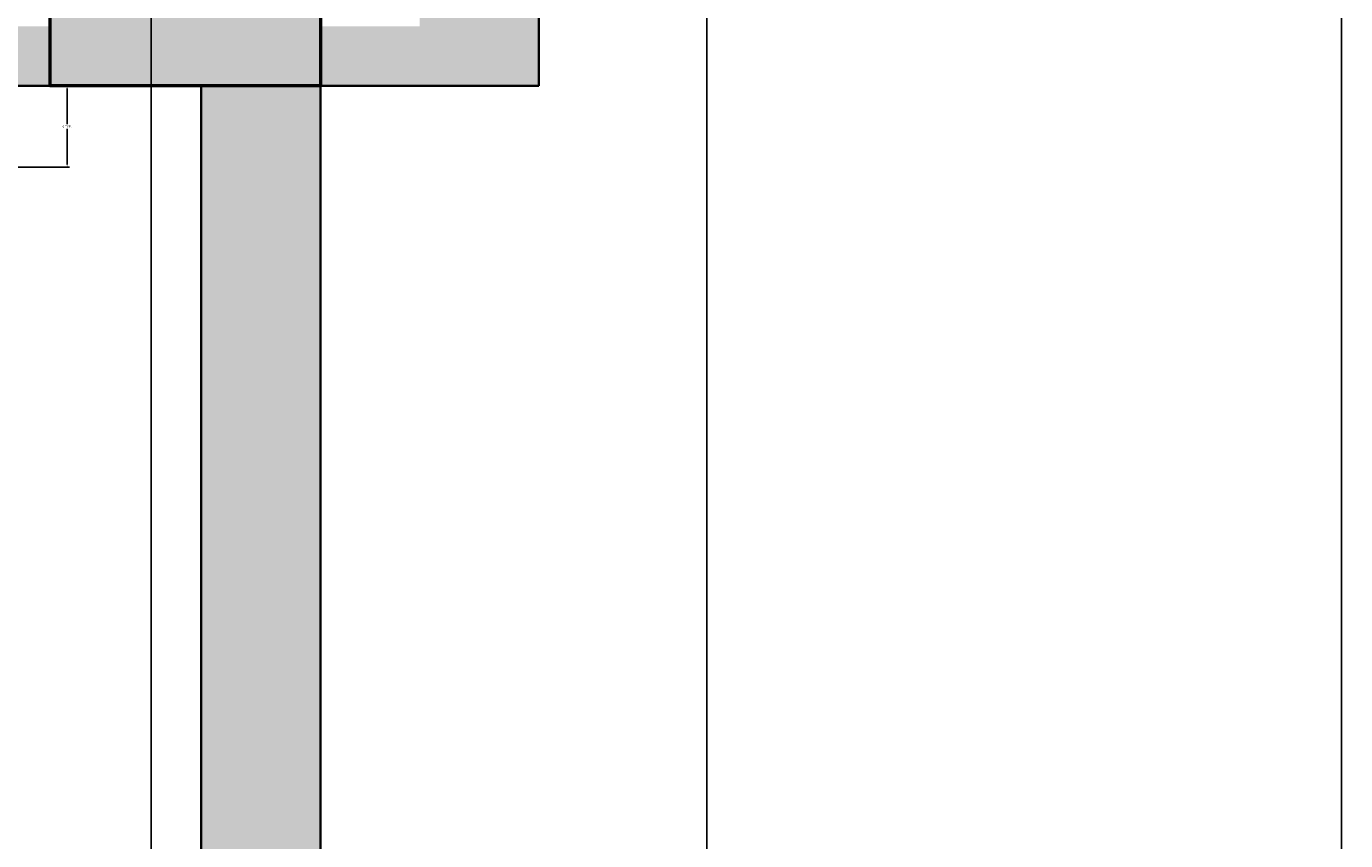
# Model space of a CAD drawing. Units: inches. Extents: x 1998 to 2588, y 1139 to 1977.
# Tile 133 of 134: x 2489 to 2588, y 1698 to 1760. Entities that reach past the tile are written whole.
import ezdxf

# ---------------------------------------------------------------- set-up
doc = ezdxf.new("R2010")
doc.units = ezdxf.units.IN
for name, color, linetype, lineweight in [('A-ANNO-DIMS', 2, 'Continuous', 18), ('A-COLS-PATT', 250, 'Continuous', 13), ('A-WALL-PATT', 252, 'Continuous', 13), ('COLUMN', 10, 'Continuous', 50), ('WALL', 200, 'Continuous', 35)]:
    doc.layers.add(name, color=color, linetype=linetype, lineweight=lineweight)
doc.styles.get("Standard").update_dxf_attribs({"font": 'arial.ttf'})
doc.dimstyles.get("Standard").update_dxf_attribs({"dimtxt": 0.18, "dimasz": 0.18, "dimexe": 0.18, "dimexo": 0.0625, "dimgap": 0.09, "dimtad": 0, "dimtih": 1, "dimtoh": 1, "dimdec": 4, "dimzin": 0, "dimdsep": 46, "dimtxsty": 'Standard', "dimcen": 0.09, "dimadec": 0, "dimazin": 0, "dimtfac": 1, "dimtdec": 4, "dimtofl": 0, "dimtmove": 0, "dimatfit": 3, "dimfxl": 1, "dimtolj": 1, "dimtzin": 0, "dimarcsym": 0})

# ---------------------------------------------------------------- blocks, each defined once
blk = doc.blocks.new('*D18')
at = {"layer": 'A-ANNO-DIMS', "color": 0, "lineweight": -2, "transparency": 16777216}
for p, q in [((2481.104, 1755.232), (2492.018, 1755.232)), ((2491.838, 1755.052), (2491.838, 1752.353)), ((2491.838, 1749.289), (2491.838, 1751.989)), ((2481.104, 1749.109), (2492.018, 1749.109))]:
    blk.add_line(p, q, dxfattribs=at)
at = {"layer": 'A-ANNO-DIMS', "color": 0, "transparency": 16777216}
for points in [[(2491.808, 1755.052), (2491.868, 1755.052), (2491.838, 1755.232)], [(2491.808, 1749.289), (2491.868, 1749.289), (2491.838, 1749.109)]]:
    blk.add_solid(points, dxfattribs=at)
at = {"layer": 'Defpoints', "color": 0, "transparency": 16777216}
for p in [(2481.042, 1755.232), (2491.838, 1755.232), (2481.042, 1749.109)]:
    blk.add_point(p, dxfattribs=at)
at = {"layer": 'A-ANNO-DIMS', "color": 0, "transparency": 16777216, "insert": (2491.838, 1752.171), "char_height": 0.18, "attachment_point": 5}
blk.add_mtext('\\A1;6 TYP.', dxfattribs=at)
blk = doc.blocks.new('*D24')
at = {"layer": 'A-ANNO-DIMS', "color": 0, "lineweight": -2, "transparency": 16777216}
for p, q in [((2398.535, 1911.232), (2588.309, 1911.232)), ((2588.129, 1911.052), (2588.129, 1570.164)), ((2588.129, 1228.912), (2588.129, 1569.8)), ((2527.535, 1228.732), (2588.309, 1228.732))]:
    blk.add_line(p, q, dxfattribs=at)
at = {"layer": 'A-ANNO-DIMS', "color": 0, "transparency": 16777216}
for points in [[(2588.099, 1911.052), (2588.159, 1911.052), (2588.129, 1911.232)], [(2588.099, 1228.912), (2588.159, 1228.912), (2588.129, 1228.732)]]:
    blk.add_solid(points, dxfattribs=at)
at = {"layer": 'Defpoints', "color": 0, "transparency": 16777216}
for p in [(2398.473, 1911.232), (2588.129, 1911.232), (2527.473, 1228.732)]:
    blk.add_point(p, dxfattribs=at)
at = {"layer": 'A-ANNO-DIMS', "color": 0, "transparency": 16777216, "insert": (2588.129, 1569.982), "char_height": 0.18, "attachment_point": 5}
blk.add_mtext('\\A1;682.5', dxfattribs=at)
blk = doc.blocks.new('*D31')
at = {"layer": 'A-ANNO-DIMS', "color": 0, "lineweight": -2, "transparency": 16777216}
for p, q in [((2498.179, 1636.795), (2498.179, 1977.362)), ((2498.359, 1977.182), (2518.957, 1977.182)), ((2539.999, 1977.182), (2519.4, 1977.182)), ((2540.179, 1636.795), (2540.179, 1977.362))]:
    blk.add_line(p, q, dxfattribs=at)
at = {"layer": 'A-ANNO-DIMS', "color": 0, "transparency": 16777216}
for points in [[(2498.359, 1977.212), (2498.359, 1977.152), (2498.179, 1977.182)], [(2539.999, 1977.212), (2539.999, 1977.152), (2540.179, 1977.182)]]:
    blk.add_solid(points, dxfattribs=at)
at = {"layer": 'Defpoints', "color": 0, "transparency": 16777216}
for p in [(2540.179, 1977.182), (2498.179, 1636.732), (2540.179, 1636.732)]:
    blk.add_point(p, dxfattribs=at)
at = {"layer": 'A-ANNO-DIMS', "color": 0, "transparency": 16777216, "insert": (2519.179, 1977.182), "char_height": 0.18, "attachment_point": 5}
blk.add_mtext('\\A1;42', dxfattribs=at)

msp = doc.modelspace()

# ---------------------------------------------------------------- hatches: boundary and pattern name
at = {"layer": 'A-COLS-PATT'}
h = msp.add_hatch(color=256, dxfattribs=at)
h.dxf.hatch_style = 1
h.paths.add_polyline_path([(2099.4125, 1888.7324), (2087.9729, 1888.7324), (2087.9729, 1868.3278), (2099.4125, 1868.3278)])
h.paths.add_polyline_path([(2234.4125, 1888.7324), (2222.9729, 1888.7324), (2222.9729, 1868.3278), (2234.4125, 1868.3278)])
h.paths.add_polyline_path([(2341.4729, 1886.637), (2330.0332, 1886.637), (2330.0332, 1866.2324), (2341.4729, 1866.2324)])
h.paths.add_polyline_path([(2507.8006, 1882.7324), (2487.396, 1882.7324), (2487.396, 1871.2927), (2507.8006, 1871.2927)])
h.paths.add_polyline_path([(2510.9729, 1766.672), (2490.5682, 1766.672), (2490.5682, 1755.2324), (2510.9729, 1755.2324)])
h.paths.add_polyline_path([(2345.9729, 1759.7324), (2334.5332, 1759.7324), (2334.5332, 1739.3278), (2345.9729, 1739.3278)])
h.paths.add_polyline_path([(2234.4125, 1774.3318), (2222.9729, 1774.3318), (2222.9729, 1753.9272), (2234.4125, 1753.9272)])
h.paths.add_polyline_path([(2099.4125, 1775.637), (2087.9729, 1775.637), (2087.9729, 1755.2324), (2099.4125, 1755.2324)])
h.paths.add_polyline_path([(2098.0956, 1593.7241), (2077.691, 1593.7241), (2077.691, 1582.2845), (2098.0956, 1582.2845)])
h.paths.add_polyline_path([(2227.4729, 1604.637), (2216.0332, 1604.637), (2216.0332, 1584.2324), (2227.4729, 1584.2324)])
h.paths.add_polyline_path([(2345.9729, 1647.5211), (2334.5332, 1647.5211), (2334.5332, 1627.1165), (2345.9729, 1627.1165)])
h.paths.add_polyline_path([(2522.3775, 1641.2324), (2501.9729, 1641.2324), (2501.9729, 1629.7927), (2522.3775, 1629.7927)])
h.paths.add_polyline_path([(2522.3775, 1480.7324), (2501.9729, 1480.7324), (2501.9729, 1469.2927), (2522.3775, 1469.2927)])
h.paths.add_polyline_path([(2345.9729, 1488.5616), (2334.5332, 1488.5616), (2334.5332, 1468.1569), (2345.9729, 1468.1569)])
h.paths.add_polyline_path([(2234.4125, 1486.137), (2227.4729, 1486.137), (2227.4729, 1465.7324), (2234.4125, 1465.7324)])
h.paths.add_polyline_path([(2227.4729, 1486.137), (2222.9729, 1486.137), (2222.9729, 1465.7324), (2227.4729, 1465.7324)])
h.paths.add_polyline_path([(2108.3775, 1470.2324), (2087.9729, 1470.2324), (2087.9729, 1458.7927), (2108.3775, 1458.7927)])
h.paths.add_polyline_path([(2096.9729, 1365.5012), (2087.9729, 1365.5012), (2087.9729, 1345.0966), (2096.9729, 1345.0966)])
h.paths.add_polyline_path([(2087.9729, 1365.5012), (2085.5332, 1365.5012), (2085.5332, 1345.0966), (2087.9729, 1345.0966)])
h.paths.add_polyline_path([(2234.4125, 1285.137), (2222.9729, 1285.137), (2222.9729, 1264.7324), (2234.4125, 1264.7324)])
h.paths.add_polyline_path([(2345.9729, 1285.137), (2334.5332, 1285.137), (2334.5332, 1264.7324), (2345.9729, 1264.7324)])
h.paths.add_polyline_path([(2503.1458, 1240.172), (2482.7412, 1240.172), (2482.7412, 1228.7324), (2503.1458, 1228.7324)])
h.paths.add_polyline_path([(2510.9729, 1369.172), (2490.5682, 1369.172), (2490.5682, 1357.7324), (2510.9729, 1357.7324)])
at = {"layer": 'A-WALL-PATT'}
h = msp.add_hatch(color=256, dxfattribs=at)
h.dxf.hatch_style = 1
h.paths.add_polyline_path([(2227.4729, 1911.2324), (2222.9729, 1911.2324), (2222.9729, 1888.7324), (2227.4729, 1888.7324)])
h.paths.add_polyline_path([(2236.4493, 1870.3636), (2236.4493, 1875.2324), (2234.4125, 1875.2324), (2234.4125, 1868.3278), (2227.4729, 1868.3278), (2227.4729, 1866.2324), (2236.4493, 1866.2324)])
h.paths.add_polyline_path([(2330.0332, 1875.2324), (2263.9907, 1875.2324), (2263.9907, 1866.2324), (2330.0332, 1866.2324)])
h.paths.add_polyline_path([(2345.9729, 1906.7324), (2393.9729, 1906.7324), (2393.9729, 1882.7324), (2345.9729, 1882.7324), (2345.9729, 1878.2324), (2393.9729, 1878.2324), (2398.4729, 1878.2324), (2398.4729, 1882.7324), (2398.4729, 1911.2324), (2345.9729, 1911.2324), (2341.4729, 1911.2324), (2341.4729, 1866.2324), (2341.4729, 1790.0412), (2345.9729, 1790.0412), (2345.9729, 1875.2324)])
h.paths.add_polyline_path([(2398.4729, 1878.2324), (2393.9729, 1878.2324), (2393.9729, 1798.2324), (2393.9729, 1793.7324), (2398.4729, 1793.7324)], flags=17)
h.paths.add_polyline_path([(2393.9729, 1798.2324), (2375.7311, 1798.2324, -0.005968), (2375.7384, 1797.6146), (2375.7384, 1793.7324), (2393.9729, 1793.7324)], flags=17)
h.paths.add_polyline_path([(2349.8569, 1797.6146), (2349.8569, 1798.2324), (2345.9729, 1798.2324), (2345.9729, 1793.7324), (2349.8569, 1793.7324)], flags=17)
h.paths.add_polyline_path([(2398.4729, 1793.7324), (2393.9729, 1793.7324), (2393.9729, 1790.0412), (2398.4729, 1790.0412)], flags=17)
h.paths.add_polyline_path([(2527.4729, 1882.7324), (2507.8006, 1882.7324), (2507.8006, 1878.2324), (2518.4729, 1878.2324), (2518.4729, 1759.7324), (2510.9729, 1759.7324), (2510.9729, 1755.2324), (2527.4729, 1755.2324)])
h.paths.add_polyline_path([(2487.396, 1882.7324), (2398.4729, 1882.7324), (2398.4729, 1878.2324), (2487.396, 1878.2324)])
h.paths.add_polyline_path([(2490.5682, 1759.7324), (2345.9729, 1759.7324), (2345.9729, 1755.2324), (2490.5682, 1755.2324)])
h.paths.add_polyline_path([(2398.4729, 1760.5844), (2398.3914, 1760.5844), (2393.9729, 1760.5844), (2393.9729, 1759.7324), (2398.4729, 1759.7324)])
h.paths.add_polyline_path([(2334.5332, 1759.7324), (2234.4125, 1759.7324), (2234.4125, 1755.2324), (2334.5332, 1755.2324)])
h.paths.add_polyline_path([(2345.9729, 1760.5844), (2341.5543, 1760.5844), (2341.4729, 1760.5844), (2341.4729, 1759.7324), (2345.9729, 1759.7324)])
h.paths.add_polyline_path([(2222.9729, 1759.7324), (2221.7204, 1759.7324), (2221.7204, 1755.2324), (2222.9729, 1755.2324)])
h.paths.add_polyline_path([(2061.4729, 1702.7324), (2059.4729, 1702.7324), (2059.4729, 1584.2324), (2061.4729, 1584.2324)])
h.paths.add_polyline_path([(2061.4729, 1584.2324), (2059.4729, 1584.2324), (2059.4729, 1470.2324), (2061.4729, 1470.2324)])
h.paths.add_polyline_path([(2510.9729, 1469.2927), (2501.9729, 1469.2927), (2501.9729, 1369.172), (2510.9729, 1369.172)])
h.paths.add_polyline_path([(2227.4729, 1369.7324), (2227.4729, 1417.7324), (2221.4126, 1417.7324), (2221.4126, 1413.2324), (2222.9729, 1413.2324), (2222.9729, 1293.2324), (2222.9729, 1285.137), (2227.4729, 1285.137)])
h = msp.add_hatch(color=256, dxfattribs=at)
h.dxf.hatch_style = 1
h.paths.add_polyline_path([(2527.4729, 1362.2324), (2510.9729, 1362.2324), (2510.9729, 1357.7324), (2518.4729, 1357.7324), (2518.4729, 1237.7324), (2503.1458, 1237.7324), (2503.1458, 1228.7324), (2527.4729, 1228.7324)])
h.paths.add_polyline_path([(2490.5682, 1362.2324), (2398.4729, 1362.2324), (2398.4729, 1357.7324), (2490.5682, 1357.7324)])
h.paths.add_polyline_path([(2224.9729, 1264.7324), (2222.9729, 1264.7324), (2222.9729, 1232.4125), (2341.4729, 1232.4125), (2341.4729, 1234.4125), (2224.9729, 1234.4125)])
h.paths.add_polyline_path([(2334.5332, 1273.7324), (2264.7638, 1273.7324), (2264.7638, 1269.5611, -0.043659), (2264.3413, 1264.7324), (2334.5332, 1264.7324)])
h.paths.add_polyline_path([(2236.9551, 1273.7324), (2234.4125, 1273.7324), (2234.4125, 1264.7324), (2236.9551, 1264.7324), (2236.9551, 1269.5611)])
h.paths.add_polyline_path([(2222.9729, 1293.2324), (2096.9729, 1293.2324), (2096.9729, 1345.0966), (2087.9729, 1345.0966), (2087.9729, 1284.2324), (2222.9729, 1284.2324), (2222.9729, 1285.137)])
h.paths.add_polyline_path([(2096.9729, 1458.7927), (2087.9729, 1458.7927), (2087.9729, 1417.7324), (2087.9729, 1413.2324), (2096.9729, 1413.2324), (2096.9729, 1417.7324)])
h.paths.add_polyline_path([(2096.9729, 1413.2324), (2087.9729, 1413.2324), (2087.9729, 1365.5012), (2096.9729, 1365.5012), (2096.9729, 1369.3358)])
h.paths.add_polyline_path([(2186.2943, 1417.7324), (2138.6074, 1417.7324), (2096.9729, 1417.7324), (2096.9729, 1413.2324), (2138.6074, 1413.2324), (2186.2943, 1413.2324)])
h.paths.add_polyline_path([(2181.4729, 1465.7324), (2176.9729, 1465.7324), (2176.9729, 1451.6434), (2181.4729, 1451.6434)])
h.paths.add_polyline_path([(2181.4729, 1422.1664), (2176.9729, 1422.1664), (2176.9729, 1417.7324), (2181.4729, 1417.7324)])
h.paths.add_polyline_path([(2063.9729, 1465.7324), (2087.9729, 1465.7324), (2087.9729, 1470.2324), (2059.4729, 1470.2324), (2059.4729, 1413.2324), (2087.9729, 1413.2324), (2087.9729, 1417.7324), (2063.9729, 1417.7324)])
h.paths.add_polyline_path([(2181.4729, 1755.2324), (2176.9729, 1755.2324), (2176.9729, 1748.6798), (2177.0513, 1748.6798), (2181.4729, 1748.6798)])
h.paths.add_polyline_path([(2227.4729, 1707.2324), (2220.4647, 1707.2324), (2220.4647, 1702.7324), (2222.9729, 1702.7324), (2222.9729, 1604.637), (2227.4729, 1604.637)])
h.paths.add_polyline_path([(2114.9729, 1702.7324), (2105.9729, 1702.7324), (2105.9729, 1628.4781, -0.0318759), (2110.1012, 1628.7416), (2114.9729, 1628.7416)])
h.paths.add_polyline_path([(2345.9729, 1739.3278), (2341.4729, 1739.3278), (2341.4729, 1647.5211), (2345.9729, 1647.5211)])
h.paths.add_polyline_path([(2350.6273, 1641.2324), (2345.9729, 1641.2324), (2345.9729, 1636.7324), (2350.6273, 1636.7324), (2350.6273, 1639.8729)])
h.paths.add_polyline_path([(2501.9729, 1641.2324), (2407.9729, 1641.2324), (2392.5005, 1641.2324), (2392.5005, 1639.8729), (2392.5005, 1636.7324), (2501.9729, 1636.7324)])
h.paths.add_polyline_path([(2510.9729, 1755.2324), (2501.9729, 1755.2324), (2501.9729, 1641.2324), (2510.9729, 1641.2324)])
h.paths.add_polyline_path([(2549.1786, 1641.2324), (2522.3775, 1641.2324), (2522.3775, 1636.7324), (2540.1786, 1636.7324), (2540.1786, 1480.7324), (2522.3775, 1480.7324), (2522.3775, 1476.2324), (2549.1786, 1476.2324)])
h.paths.add_polyline_path([(2498.1786, 1594.7324), (2407.9729, 1594.7324), (2407.9729, 1585.7324), (2416.9729, 1585.7324), (2489.1786, 1585.7324), (2489.1786, 1531.7324), (2416.9729, 1531.7324), (2407.9729, 1531.7324), (2407.9729, 1522.7324), (2498.1786, 1522.7324)])
h.paths.add_polyline_path([(2351.6437, 1480.7324), (2345.9729, 1480.7324), (2345.9729, 1476.2324), (2351.6437, 1476.2324), (2351.6437, 1477.5919)])
h.paths.add_polyline_path([(2501.9729, 1480.7324), (2498.1786, 1480.7324), (2407.9729, 1480.7324), (2393.5168, 1480.7324), (2393.5168, 1477.5919), (2393.5168, 1476.2324), (2501.9729, 1476.2324)])

# ---------------------------------------------------------------- linework, layer by layer
at = {"layer": 'COLUMN'}
msp.add_lwpolyline([(2510.9729, 1766.672), (2510.9729, 1755.2324), (2490.5682, 1755.2324), (2490.5682, 1766.672)], close=True, dxfattribs=at)
at = {"layer": 'WALL'}
for p, q in [((2527.4729, 1882.7324), (2527.4729, 1755.2324)), ((2345.9729, 1755.2324), (2527.4729, 1755.2324)), ((2345.9729, 1755.2324), (2501.9729, 1755.2324)), ((2501.9729, 1755.2324), (2501.9729, 1641.2324)), ((2510.9729, 1755.2324), (2510.9729, 1641.2324))]:
    msp.add_line(p, q, dxfattribs=at)

# ---------------------------------------------------------------- dimensions: what is measured, and where the dimension line sits
at = {"layer": 'A-ANNO-DIMS'}
dim = msp.add_linear_dim(base=(2540.1786, 1977.1824), p1=(2498.1786, 1636.7324), p2=(2540.1786, 1636.7324), dimstyle='Standard', override={"dimdec": 0, "dimlfac": 1, "dimrnd": 0, "dimzin": 0, "dimdsep": 46, "dimlunit": 2}, dxfattribs=at)
dim.commit()
dim.dimension.update_dxf_attribs({"geometry": '*D31', "text_midpoint": (2519.1786, 1977.1824)})
dim = msp.add_linear_dim(base=(2588.1286, 1911.2324), p1=(2527.4729, 1228.7324), p2=(2398.4729, 1911.2324), angle=90, dimstyle='Standard', override={"dimdec": 1, "dimlfac": 1, "dimrnd": 0, "dimzin": 0, "dimdsep": 46, "dimlunit": 2}, dxfattribs=at)
dim.commit()
dim.dimension.update_dxf_attribs({"geometry": '*D24', "text_midpoint": (2588.1286, 1569.9824)})
dim = msp.add_linear_dim(base=(2491.8385, 1755.2324), p1=(2481.0415, 1749.1089), p2=(2481.0415, 1755.2324), angle=90, text='<> TYP.', dimstyle='Standard', override={"dimdec": 0, "dimlfac": 1, "dimrnd": 0, "dimzin": 0, "dimdsep": 46, "dimlunit": 2}, dxfattribs=at)
dim.commit()
dim.dimension.update_dxf_attribs({"geometry": '*D18', "text_midpoint": (2491.8385, 1752.1707)})

doc.saveas('drawing.dxf')
